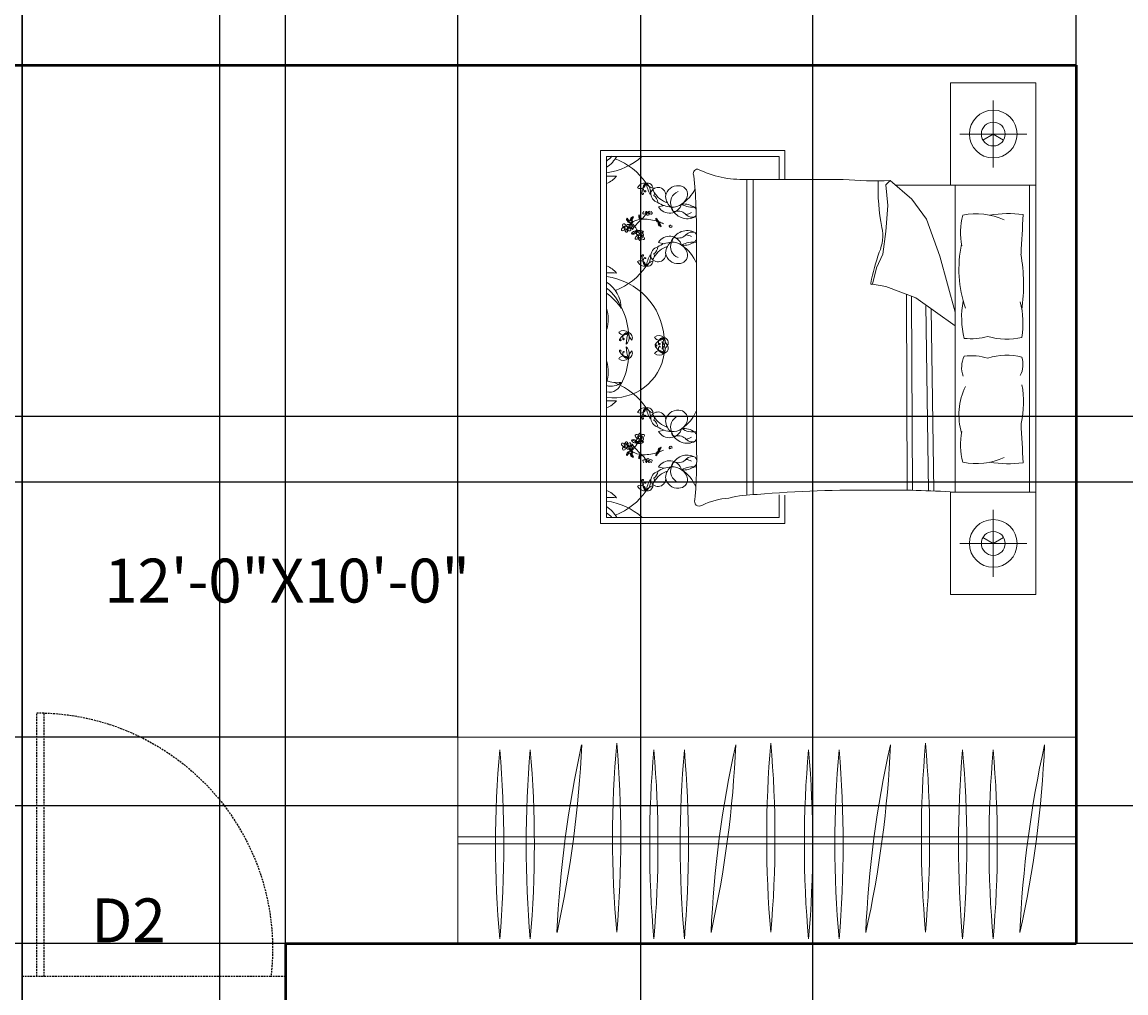
# Model space of a CAD drawing. Units: inches. Extents: x 3 to 576, y -689 to 51.
# Tile 15 of 21: x 111 to 262, y -261 to -128. Entities that reach past the tile are written whole.
import ezdxf

# ---------------------------------------------------------------- set-up
doc = ezdxf.new("R2010")
doc.units = ezdxf.units.IN
doc.header["$MEASUREMENT"] = 0
doc.linetypes.add('DASHED2', pattern=[0.375, 0.25, -0.125])
for name, color, linetype, lineweight in [('A-ANNO-DIMS', 2, 'Continuous', 18), ('A-ANNO-TEXT', 3, 'Continuous', 18), ('A-AREA-IDEN', 7, 'Continuous', 18), ('A-DOOR', 4, 'DASHED2', 25), ('A-FURN', 8, 'Continuous', 18), ('A-WALL', 7, 'Continuous', 50)]:
    doc.layers.add(name, color=color, linetype=linetype, lineweight=lineweight)
doc.styles.get("Standard").update_dxf_attribs({"font": 'arial.ttf'})
doc.dimstyles.get("Standard").update_dxf_attribs({"dimtxt": 0.18, "dimasz": 0.18, "dimexe": 0.18, "dimexo": 0.0625, "dimgap": 0.09, "dimtad": 0, "dimtih": 1, "dimtoh": 1, "dimdec": 0, "dimzin": 0, "dimdsep": 46, "dimlunit": 3, "dimtxsty": 'Standard', "dimcen": 0.09, "dimadec": 0, "dimazin": 0, "dimtfac": 1, "dimtdec": 0, "dimtofl": 0, "dimtmove": 0, "dimatfit": 3, "dimfxl": 1, "dimtolj": 1, "dimtzin": 0, "dimarcsym": 0})

# ---------------------------------------------------------------- blocks, each defined once
blk = doc.blocks.new('BED-DOUBLE')
for p, q in [((59.45, 69.91), (59.45, 0)), ((53.63, 58.35), (53.63, 67.49)), ((49.06, 62.92), (58.2, 62.92)), ((0, 60.68), (25.18, 60.68)), ((0, 9.72), (0, 60.68)), ((25.18, 60.68), (25.18, 56.73)), ((0.81, 59.87), (0.81, 10.53)), ((24.37, 59.87), (0.81, 59.87)), ((24.37, 56.73), (24.37, 59.87)), ((19.95, 13.6), (19.95, 56.73)), ((20.82, 13.66), (20.82, 56.73)), ((38.97, 55.99), (39.54, 56.55)), ((39.25, 53.16), (38.97, 55.99)), ((39.54, 56.55), (42.51, 54.01)), ((59.45, 55.93), (40.27, 55.93)), ((48.41, 55.93), (48.41, 13.98)), ((58.56, 13.98), (58.56, 55.93)), ((7.9, 52.98), (8.69, 53.14)), ((38.97, 49.62), (39.25, 53.16)), ((42.51, 54.01), (44.49, 51.31)), ((44.49, 51.31), (46.33, 46.22)), ((13.08, 20.76), (13.08, 49.15)), ((38.55, 46.5), (38.97, 49.62)), ((7.9, 48.1), (8.69, 47.94)), ((37.7, 44.66), (38.55, 46.5)), ((46.33, 46.22), (48.41, 38.59)), ((37.13, 42.39), (37.7, 44.66)), ((38.97, 42.11), (37.13, 42.39)), ((43.07, 40.55), (38.97, 42.11)), ((41.87, 14.23), (41.76, 41.05)), ((42.58, 14.23), (42.48, 40.78)), ((48.41, 36.72), (43.07, 40.55)), ((44.78, 14.2), (44.43, 39.58)), ((45.5, 14.17), (45.15, 39.06)), ((7.9, 22.3), (8.69, 22.46)), ((7.9, 17.41), (8.69, 17.26)), ((24.37, 10.53), (24.37, 13.61)), ((25.18, 13.59), (25.18, 9.72)), ((53.63, 11.56), (53.63, 2.42)), ((25.18, 9.72), (0, 9.72)), ((0.81, 10.53), (24.37, 10.53)), ((49.06, 6.99), (58.2, 6.99))]:
    blk.add_line(p, q)
for points in [[(47.8, 55.93), (47.8, 69.91), (59.45, 69.91)], [(53.63, 62.92), (52.22, 62.1)], [(53.63, 62.92), (55.04, 62.1)], [(59.45, 13.98), (47.8, 13.98), (47.8, 0), (59.45, 0)], [(53.63, 6.99), (52.22, 7.81)], [(53.63, 6.99), (55.04, 7.81)]]:
    blk.add_lwpolyline(points)
for points in [[(33.13, 56.7, 0.001242), (19.87, 56.73, -0.127202), (13.26, 58.14)], [(57.71, 51.91, 0.074897), (53.14, 51.83, -0.472817)], [(52.89, 35.28, 0.14099), (57.55, 35.14, 0.235245)], [(52.89, 32.3, -0.14099), (57.55, 32.44, -0.235245)], [(57.71, 18, -0.074897), (53.14, 18.08, 0.472817)], [(21.37, 13.68, 0.056112), (17.53, 13.18, 0.095341), (13.82, 12.19)]]:
    blk.add_lwpolyline(points, format="xyb")
for centre, radius in [((53.63, 62.92), 3.26), ((53.63, 62.92), 1.63), ((3.49, 50.11), 0.178), ((5.36, 48.94), 0.178), ((5.36, 21.45), 0.178), ((3.49, 20.29), 0.178), ((53.63, 6.99), 3.26), ((53.63, 6.99), 1.63)]:
    blk.add_circle(centre, radius)
for centre, radius, start, end in [((-2.47, 63.69), 5.54, 306.3036, 316.4814), ((-1.64, 62.09), 4.45, 303.4617, 330.1116), ((-0.42, 66.67), 9.13, 277.745, 311.8856), ((-1.32, 51.05), 9.13, 34.3865, 68.5908), ((13.3, 57.49), 0.645, 93.98, 207.3412), ((-0.61, 59.6), 3.71, 292.5547, 318.9546), ((1.38, 69.77), 12.63, 267.4081, 273.6519), ((6, 55.22), 1.01, 77.7115, 159.0387), ((5.45, 56.23), 0.762, 238.4633, 358.2869), ((7.95, 54.69), 2.31, 138.8402, 177.9352), ((6.56, 55.55), 0.747, 117.6827, 223.7762), ((6.39, 55.47), 0.757, 2.9516, 103.728), ((12.45, 57.59), 6.39, 192.5173, 207.1824), ((5.37, 55.04), 1.44, 345.4653, 54.2343), ((7.54, 57.02), 1.56, 211.3827, 255.2969), ((10.53, 54.2), 1.67, 84.9449, 172.8857), ((10.7, 54.68), 1.18, 354.4856, 91.0538), ((-59.69, 49.98), 72.78, 359.3433, 5.6887), ((37.8, 120.65), 64.12, 265.8294, 271.553), ((64.29, 55.36), 26.39, 177.4519, 191.3392), ((5.76, 54.77), 0.113, 177.9352, 11.4834), ((5.81, 54.78), 0.0551, 11.4834, 127.9409), ((6.09, 55.1), 0.0988, 223.7762, 159.7183), ((7.84, 54.58), 1.05, 350.264, 160.8688), ((8.16, 54.83), 1.31, 175.969, 254.3045), ((6.7, 54.8), 0.643, 333.9755, 53.2681), ((6.41, 53.42), 1.4, 6.1662, 51.5825), ((10.15, 56.66), 3.3, 211.2614, 251.7045), ((10.9, 54.49), 2.03, 182.3591, 234.0401), ((11.17, 53.54), 1.62, 111.5819, 201.4221), ((9.83, 55.04), 2.1, 265.2933, 346.921), ((8.16, 57.76), 5.29, 303.6671, 333.2997), ((9.88, 56.69), 3.75, 236.2883, 266.5076), ((9.4, 53.85), 1.74, 209.9085, 343.1337), ((10.13, 52.75), 0.434, 167.3041, 285.1471), ((11.31, 50.67), 2.7, 122.7011, 126.3445), ((11.81, 53.58), 2.23, 199.2822, 299.1751), ((12.57, 55.82), 2.9, 238.8218, 279.1554), ((11.31, 50.67), 2.7, 55.785, 94.7304), ((12.31, 52.24), 0.842, 30.0293, 52.325), ((3.75, 51.26), 0.199, 124.3538, 214.3923), ((4.17, 51.39), 0.538, 176.9701, 248.2913), ((8.01, 54.23), 5.2, 212.6784, 216.3746), ((4.48, 51.12), 0.464, 122.8155, 187.3992), ((4.69, 51.06), 0.538, 109.4799, 177.6828), ((4.4, 51.4), 0.199, 56.8636, 146.9021), ((4.5, 51.18), 0.206, 148.8844, 224.2646), ((8.78, 48.6), 5.2, 145.1882, 148.8844), ((5.81, 48.38), 2.9, 94.756, 119.2041), ((11.99, 44.2), 9.55, 132.2412, 142.1744), ((7.17, 51.8), 1.97, 178.3264, 187.1302), ((5.04, 51.53), 0.367, 11.3256, 64.4621), ((6.29, 52.06), 1.1, 190.2588, 210.656), ((5.55, 51.61), 0.336, 188.3432, 274.2869), ((5.84, 51.79), 0.586, 210.656, 242.6341), ((6.28, 52.3), 1.12, 218.2101, 226.3071), ((5.45, 51.35), 0.142, 325.7657, 67.4417), ((1.03, 56.11), 6.64, 313.1541, 322.0459), ((5.96, 45.49), 5.79, 73.5842, 93.8277), ((5.91, 52.13), 0.137, 142.4737, 265.053), ((6.09, 52.15), 0.294, 127.7621, 169.0403), ((5.94, 52.4), 0.414, 265.053, 338.3618), ((6.48, 51.84), 0.541, 113.4276, 137.6104), ((6.42, 52.4), 0.178, 183.2768, 356.7232), ((6.55, 52.07), 0.291, 139.7889, 227.6792), ((6.46, 51.97), 0.153, 227.6792, 350.3487), ((5.87, 52.08), 0.583, 353.0852, 15.7171), ((6.25, 52.01), 0.368, 350.3487, 43.6538), ((6.93, 52.39), 0.428, 198.7263, 262.5032), ((6.59, 52.19), 0.17, 1.1081, 91.8675), ((6.91, 52.1), 0.138, 255.2356, 54.9248), ((6.7, 52.15), 0.297, 11.5637, 52.6358), ((9.52, 51.39), 1.97, 178.3264, 187.1302), ((7.39, 51.11), 0.367, 11.3256, 64.4621), ((8.64, 51.64), 1.1, 190.2588, 210.656), ((10.62, 50.95), 1.43, 41.5653, 105.1471), ((11.41, 53.92), 2.01, 277.436, 299.9149), ((12.48, 52.59), 1.05, 221.5653, 293.8354), ((12.31, 52.24), 0.842, 314.4517, 333.558), ((58.53, 49.42), 9.37, 165.1039, 191.0369), ((51.31, 43.01), 9.01, 65.1316, 101.7583), ((723.03, 13.38), 666.43, 176.68521, 177.14978), ((2.98, 49.84), 0.137, 142.4737, 265.053), ((3.16, 49.87), 0.294, 61.2196, 169.0403), ((3, 50.12), 0.414, 265.053, 338.3618), ((3.35, 50.47), 0.351, 157.4086, 261.4386), ((3.15, 50.48), 0.176, 58.0499, 135.6268), ((3.55, 49.55), 0.541, 113.4276, 137.6104), ((3.34, 50.37), 0.118, 172.906, 277.132), ((2.95, 50.16), 0.561, 14.7558, 58.0499), ((3.62, 49.79), 0.291, 139.7889, 227.6792), ((3.74, 50.31), 0.243, 36.1046, 181.4281), ((2.93, 49.79), 0.583, 353.0852, 15.7171), ((4.04, 51.23), 0.464, 190.3057, 287.1958), ((3.31, 49.72), 0.368, 350.3487, 43.6538), ((3.59, 50.5), 0.245, 270.0645, 331.1507), ((3.8, 50.44), 0.28, 221.8413, 265.7877), ((4, 50.1), 0.428, 198.7263, 262.5032), ((3.66, 49.9), 0.17, 1.1081, 91.8675), ((3.8, 50.33), 0.174, 263.7526, 41.7054), ((3.76, 49.86), 0.297, 11.5637, 86.365), ((3.99, 51.27), 0.206, 216.3746, 291.7548), ((5.81, 48.38), 2.9, 124.0033, 132.4917), ((3.98, 49.81), 0.138, 255.2356, 54.9248), ((2.83, 48.01), 3.1, 63.7819, 68.2913), ((4.48, 50.4), 0.493, 128.3208, 208.8162), ((4.57, 50.43), 0.59, 207.7043, 254.3516), ((4.12, 50.93), 0.155, 289.3605, 111.7548), ((4.24, 50.93), 0.155, 221.8703, 44.2646), ((4.94, 50.48), 0.812, 157.2305, 229.0635), ((4.67, 50.75), 0.478, 174.4544, 220.6188), ((4.19, 50.1), 0.812, 270.278, 342.111), ((1.96, 48.08), 3.48, 30.544, 49.818), ((3.87, 50.06), 0.574, 340.0041, 40.6188), ((4.57, 50.12), 0.478, 278.7227, 324.8872), ((5.45, 49.87), 0.493, 182.8499, 266.1226), ((5.26, 50.22), 0.478, 231.7607, 277.9252), ((5.63, 50.31), 0.812, 214.5369, 286.3699), ((7.9, 51.19), 0.336, 188.3432, 274.2869), ((8.19, 51.38), 0.586, 210.656, 242.6341), ((8.64, 51.88), 1.12, 218.2101, 226.3071), ((7.81, 50.93), 0.142, 325.7657, 67.4417), ((8.21, 50.67), 0.336, 147.5332, 233.4768), ((7.94, 50.71), 0.142, 354.3784, 96.0543), ((8.51, 50.85), 0.586, 179.1859, 211.164), ((5.96, 45.49), 5.79, 63.0032, 69.8941), ((8.95, 51.12), 1.1, 211.164, 231.5612), ((9.15, 52.01), 1.97, 234.6898, 243.4936), ((9.16, 51), 1.12, 195.5129, 203.6099), ((7.9, 50.27), 0.367, 357.3579, 50.4944), ((9.48, 50.34), 0.135, 12.7051, 190.4384), ((9.56, 50.36), 0.219, 190.4384, 10.4136), ((32.84, 49.05), 5.69, 336.2616, 11.3392), ((3.53, 49.68), 0.153, 227.6792, 350.3487), ((4.73, 49.08), 0.574, 98.7227, 159.3375), ((4.44, 49.82), 0.59, 244.9899, 291.6373), ((4.49, 49.73), 0.493, 290.5253, 358.5375), ((4.85, 48.67), 0.137, 142.4737, 265.053), ((5.03, 48.7), 0.294, 61.2196, 169.0403), ((4.88, 48.95), 0.414, 265.053, 338.3618), ((5.23, 49.31), 0.351, 157.4086, 261.4386), ((5.03, 49.32), 0.176, 58.0499, 135.6268), ((5.43, 48.38), 0.541, 113.4276, 137.6104), ((5.21, 49.21), 0.118, 172.906, 277.132), ((4.83, 48.99), 0.561, 14.7558, 58.0499), ((1.96, 48.08), 3.48, 23.0501, 23.8477), ((5.5, 48.62), 0.291, 139.7889, 227.6792), ((5.4, 48.52), 0.153, 227.6792, 350.3487), ((5.4, 49.18), 0.574, 37.3105, 97.9252), ((5.61, 49.14), 0.243, 36.1046, 181.4281), ((4.81, 48.63), 0.583, 353.0852, 15.7171), ((5.47, 49.97), 0.59, 265.0106, 311.658), ((1.96, 48.08), 3.48, 357.1071, 4.7585), ((5.19, 48.56), 0.368, 350.3487, 43.6538), ((5.47, 49.33), 0.245, 270.0645, 331.1507), ((5.68, 49.27), 0.28, 221.8413, 265.7877), ((5.87, 48.94), 0.428, 198.7263, 262.5032), ((5.53, 48.74), 0.17, 1.1081, 91.8675), ((5.68, 49.17), 0.174, 263.7526, 41.7054), ((5.64, 48.7), 0.297, 11.5637, 86.365), ((5.85, 48.65), 0.138, 255.2356, 54.9248), ((9.4, 47.23), 1.74, 16.8663, 150.0915), ((10.13, 48.33), 0.434, 74.8529, 192.6959), ((11.81, 47.5), 2.23, 60.8249, 160.7178), ((10.62, 50.13), 1.43, 254.8529, 318.4347), ((11.41, 47.16), 2.01, 60.0851, 82.564), ((12.48, 48.49), 1.05, 66.1646, 138.4347), ((12.31, 48.84), 0.842, 307.675, 336.7144), ((12.31, 48.84), 0.842, 23.229, 45.5483), ((8.16, 46.25), 1.31, 105.6955, 184.031), ((6.41, 47.66), 1.4, 308.4175, 353.8338), ((10.15, 44.42), 3.3, 108.2955, 148.7386), ((9.88, 44.39), 3.75, 93.4924, 123.7117), ((10.9, 46.59), 2.03, 125.9599, 177.6409), ((11.17, 47.54), 1.62, 158.5779, 248.4181), ((9.83, 46.04), 2.1, 13.079, 94.7067), ((11.31, 50.41), 2.7, 233.6555, 237.2989), ((12.57, 45.26), 2.9, 79.7133, 121.1782), ((11.31, 50.41), 2.7, 265.2696, 304.215), ((8.16, 43.32), 5.29, 21.4941, 56.3329), ((63.55, 37.54), 27.11, 160.1194, 169.3383), ((65.19, 44.49), 16.25, 168.0397, 199.2615), ((5.45, 44.85), 0.762, 1.7131, 121.5367), ((6, 45.86), 1.01, 200.9613, 282.2885), ((5.76, 46.31), 0.113, 348.5166, 182.0648), ((7.95, 46.39), 2.31, 182.0648, 221.1598), ((5.81, 46.3), 0.0551, 232.0591, 348.5166), ((6.56, 45.54), 0.747, 136.2238, 242.3173), ((6.13, 45.97), 0.0595, 200.2667, 136.2271), ((5.37, 46.05), 1.44, 305.7657, 14.5347), ((12.45, 43.49), 6.39, 152.8176, 167.4827), ((6.39, 45.61), 0.757, 256.272, 357.0484), ((7.54, 44.06), 1.56, 104.7031, 148.6173), ((7.84, 46.5), 1.05, 199.1312, 9.736), ((6.7, 46.28), 0.643, 306.7319, 26.0245), ((10.53, 46.88), 1.67, 187.1143, 275.0551), ((10.7, 46.4), 1.18, 268.9462, 5.5144), ((32.41, 42.33), 25.35, 352.2196, 9.497), ((-0.61, 41.48), 3.71, 41.0454, 67.4453), ((1.38, 31.32), 12.63, 86.3481, 92.5919), ((-1.32, 50.03), 9.13, 291.4092, 325.6135), ((-0.42, 34.41), 9.13, 4.4623, 82.255), ((-1.64, 38.99), 4.45, 1.272, 56.5383), ((37.07, 42.55), 0.169, 178.8623, 289.7536), ((-2.47, 37.39), 5.54, 17.8504, 53.6964), ((-4.03, 34.48), 8.25, 34.0123, 54.053), ((-5.31, 35.11), 9.13, 4.4623, 27.4146), ((61.64, 37.91), 12.33, 169.8617, 193.6238), ((45.23, 36.98), 12.46, 351.5249, 13.96), ((-3.99, 37.66), 5.02, 343.5431, 17.0202), ((-6.58, 35.67), 7.42, 4.3787, 5.6357), ((-11.66, 31.77), 13.27, 19.7217, 19.9028), ((3.11, 35.07), 1.01, 47.7873, 129.1145), ((3.14, 36.22), 0.762, 208.5391, 328.3627), ((2.68, 34.8), 0.113, 148.011, 341.5592), ((4.54, 33.64), 2.31, 108.9159, 148.011), ((2.73, 34.78), 0.0551, 341.5592, 98.0167), ((3.76, 35.07), 0.747, 87.7585, 193.852), ((3.13, 34.92), 0.0988, 193.852, 129.9245), ((9.89, 33.91), 6.39, 162.593, 177.2582), ((2.48, 35.23), 1.44, 315.5411, 24.3101), ((5.35, 35.86), 1.56, 181.4585, 225.3727), ((3.58, 35.09), 0.757, 333.0274, 73.8037), ((8, 34.37), 1.01, 47.7873, 129.1145), ((8.03, 35.52), 0.762, 208.5391, 328.3627), ((9.43, 32.94), 2.31, 108.9159, 148.011), ((8.65, 34.38), 0.747, 87.7585, 193.852), ((7.37, 34.53), 1.44, 315.5411, 24.3101), ((14.78, 33.21), 6.39, 162.593, 177.2582), ((8.47, 34.4), 0.757, 333.0274, 73.8037), ((10.24, 35.16), 1.56, 181.4585, 225.3727), ((50.55, 43.52), 8.57, 264.0129, 285.8293), ((2.68, 33.27), 0.113, 18.4408, 211.989), ((4.54, 34.43), 2.31, 211.989, 251.0841), ((2.73, 33.29), 0.0551, 261.9833, 18.4408), ((3.76, 32.99), 0.747, 166.148, 272.2415), ((3.17, 33.16), 0.0595, 230.1909, 166.0209), ((9.89, 34.16), 6.39, 182.7418, 197.407), ((2.48, 32.84), 1.44, 335.6899, 44.4589), ((5.35, 32.21), 1.56, 134.6273, 178.5415), ((3.58, 32.97), 0.757, 286.1963, 26.9726), ((8.03, 32.55), 0.762, 31.6373, 151.4609), ((7.57, 34.1), 0.113, 148.011, 341.5592), ((7.57, 33.97), 0.113, 18.4408, 211.989), ((9.43, 35.13), 2.31, 211.989, 251.0841), ((7.62, 34.08), 0.0551, 341.5592, 98.0167), ((7.62, 33.99), 0.0551, 261.9833, 18.4408), ((8.65, 33.69), 0.747, 166.148, 272.2415), ((8.02, 34.22), 0.0988, 193.852, 129.9245), ((8.06, 33.86), 0.0595, 230.1909, 166.0209), ((7.37, 33.54), 1.44, 335.6899, 44.4589), ((14.78, 34.86), 6.39, 182.7418, 197.407), ((8.47, 33.67), 0.757, 286.1963, 26.9726), ((10.24, 32.91), 1.56, 134.6273, 178.5415), ((1.69, 33.95), 7.07, 262.8636, 351.8197), ((-3.99, 30.4), 5.02, 342.9798, 16.4569), ((-6.58, 32.39), 7.42, 354.3643, 355.6213), ((-11.66, 36.3), 13.27, 340.0972, 340.2783), ((3.14, 31.85), 0.762, 31.6373, 151.4609), ((3.11, 33), 1.01, 230.8855, 312.2127), ((-5.31, 32.96), 9.13, 332.5854, 355.5377), ((8, 33.7), 1.01, 230.8855, 312.2127), ((53.02, 31.01), 3.71, 155.0183, 198.5407), ((50.55, 24.06), 8.57, 74.1707, 95.9871), ((54.23, 31.48), 3.46, 333.3437, 16.1026), ((2.33, 33.04), 4.09, 248.117, 276.6195), ((1.2, 29.29), 1.64, 256.3898, 349.0739), ((1.42, 30.52), 2.07, 252.8609, 311.9049), ((-1.32, 20.37), 9.13, 34.3865, 68.5908), ((45.48, 26.29), 12.29, 346.3427, 11.1841), ((57.84, 24.53), 8.9, 153.8761, 196.1746), ((1.38, 39.08), 12.63, 267.4081, 273.6519), ((-0.61, 28.92), 3.71, 292.5547, 318.9546), ((6, 24.53), 1.01, 77.7115, 159.0387), ((5.45, 25.55), 0.762, 238.4633, 358.2869), ((7.95, 24), 2.31, 138.8402, 177.9352), ((5.81, 24.09), 0.0551, 11.4834, 127.9409), ((6.56, 24.86), 0.747, 117.6827, 223.7762), ((6.09, 24.41), 0.0988, 223.7762, 159.7183), ((6.39, 24.79), 0.757, 2.9516, 103.728), ((7.54, 26.34), 1.56, 211.3827, 255.2969), ((5.37, 24.35), 1.44, 345.4653, 54.2343), ((12.45, 26.91), 6.39, 192.5173, 207.1824), ((7.84, 23.9), 1.05, 350.264, 160.8688), ((8.16, 24.15), 1.31, 175.969, 254.3045), ((6.7, 24.12), 0.643, 333.9755, 53.2681), ((10.15, 25.98), 3.3, 211.2614, 251.7045), ((10.53, 23.52), 1.67, 84.9449, 172.8857), ((11.17, 22.86), 1.62, 111.5819, 201.4221), ((10.7, 24), 1.18, 354.4856, 91.0538), ((8.16, 27.08), 5.29, 303.6671, 338.5059), ((5.76, 24.08), 0.113, 177.9352, 11.4834), ((6.41, 22.74), 1.4, 6.1662, 51.5825), ((9.88, 26.01), 3.75, 236.2883, 266.5076), ((9.4, 23.17), 1.74, 209.9085, 343.1337), ((10.9, 23.81), 2.03, 182.3591, 234.0401), ((9.83, 24.36), 2.1, 265.2933, 346.921), ((12.57, 25.14), 2.9, 238.8218, 280.2867), ((11.31, 19.99), 2.7, 55.785, 94.7304), ((723.03, 56.53), 666.43, 182.85022, 183.31479), ((4.44, 20.58), 0.59, 68.3627, 115.0101), ((4.19, 20.3), 0.812, 17.889, 89.722), ((4.73, 21.32), 0.574, 200.6625, 261.2773), ((4.49, 20.66), 0.493, 1.4625, 69.4747), ((4.85, 21.72), 0.137, 94.947, 217.5263), ((5.03, 21.7), 0.294, 190.9597, 298.7804), ((4.88, 21.45), 0.414, 21.6382, 94.947), ((5.23, 21.09), 0.351, 98.5614, 202.5914), ((5.43, 22.01), 0.541, 222.3896, 246.5724), ((5.21, 21.19), 0.118, 82.868, 187.094), ((4.83, 21.41), 0.561, 301.9501, 345.2442), ((5.5, 21.78), 0.291, 132.3208, 220.2111), ((5.4, 21.88), 0.153, 9.6513, 132.3208), ((4.81, 21.77), 0.583, 344.2829, 6.9148), ((5.61, 21.26), 0.243, 178.5719, 323.8954), ((1.96, 22.32), 3.48, 355.2415, 2.8929), ((5.19, 21.84), 0.368, 316.3462, 9.6513), ((5.87, 21.46), 0.428, 97.4968, 161.2737), ((5.68, 21.12), 0.28, 94.2123, 138.1587), ((5.47, 21.07), 0.245, 28.8493, 89.9355), ((5.53, 21.66), 0.17, 268.1325, 358.8919), ((5.64, 21.7), 0.297, 273.635, 348.4363), ((5.68, 21.23), 0.174, 318.2946, 96.2474), ((5.85, 21.75), 0.138, 305.0752, 104.7644), ((10.13, 22.07), 0.434, 167.3041, 285.1471), ((11.31, 19.99), 2.7, 122.7011, 126.3445), ((11.81, 22.9), 2.23, 199.2822, 299.1751), ((10.62, 20.26), 1.43, 41.5653, 105.1471), ((11.41, 23.23), 2.01, 277.436, 299.9149), ((12.48, 21.91), 1.05, 221.5653, 293.8354), ((12.31, 21.55), 0.842, 23.2856, 52.325), ((12.31, 21.55), 0.842, 314.4517, 336.7144), ((58.53, 20.49), 9.37, 168.9631, 194.8961), ((2.98, 20.56), 0.137, 94.947, 217.5263), ((3.16, 20.53), 0.294, 190.9597, 298.7804), ((3, 20.28), 0.414, 21.6382, 94.947), ((3.35, 19.93), 0.351, 98.5614, 202.5914), ((3.15, 19.91), 0.176, 224.3732, 301.9501), ((3.55, 20.85), 0.541, 222.3896, 246.5724), ((3.34, 20.03), 0.118, 82.868, 187.094), ((2.95, 20.24), 0.561, 301.9501, 345.2442), ((3.62, 20.61), 0.291, 132.3208, 220.2111), ((3.53, 20.71), 0.153, 9.6513, 132.3208), ((2.93, 20.61), 0.583, 344.2829, 6.9148), ((3.74, 20.09), 0.243, 178.5719, 323.8954), ((3.31, 20.68), 0.368, 316.3462, 9.6513), ((4.04, 19.17), 0.464, 72.8042, 169.6943), ((4, 20.3), 0.428, 97.4968, 161.2737), ((3.8, 19.96), 0.28, 94.2123, 138.1587), ((3.59, 19.9), 0.245, 28.8493, 89.9355), ((3.66, 20.5), 0.17, 268.1325, 358.8919), ((3.76, 20.54), 0.297, 273.635, 348.4363), ((3.8, 20.07), 0.174, 318.2946, 96.2474), ((5.81, 22.02), 2.9, 227.5083, 235.9967), ((3.98, 20.59), 0.138, 305.0752, 104.7644), ((2.83, 22.39), 3.1, 291.7087, 296.2181), ((4.48, 20), 0.493, 151.1838, 231.6792), ((4.57, 19.96), 0.59, 105.6484, 152.2957), ((4.12, 19.47), 0.155, 248.2452, 70.6395), ((4.94, 19.92), 0.812, 130.9365, 202.7695), ((4.24, 19.47), 0.155, 315.7354, 138.1297), ((4.67, 19.65), 0.478, 139.3812, 185.5456), ((1.96, 22.32), 3.48, 310.182, 329.456), ((3.87, 20.33), 0.574, 319.3812, 19.9959), ((11.99, 26.2), 9.55, 217.8256, 227.7588), ((4.57, 20.28), 0.478, 35.1128, 81.2773), ((5.03, 21.08), 0.176, 224.3732, 301.9501), ((5.45, 20.52), 0.493, 93.8774, 177.1501), ((5.63, 20.09), 0.812, 73.6301, 145.4631), ((5.26, 20.18), 0.478, 82.0748, 128.2393), ((1.96, 22.32), 3.48, 336.1523, 336.9499), ((5.4, 21.22), 0.574, 262.0748, 322.6895), ((5.47, 20.43), 0.59, 48.342, 94.9894), ((8.21, 19.72), 0.336, 126.5232, 212.4668), ((8.51, 19.55), 0.586, 148.836, 180.8141), ((7.94, 19.68), 0.142, 263.9457, 5.6216), ((5.96, 24.9), 5.79, 290.1059, 296.9968), ((8.95, 19.28), 1.1, 128.4388, 148.836), ((9.15, 18.38), 1.97, 116.5064, 125.3102), ((9.16, 19.4), 1.12, 156.3901, 164.4871), ((7.9, 20.13), 0.367, 309.5056, 2.6421), ((9.56, 20.04), 0.219, 349.5864, 169.5616), ((9.48, 20.06), 0.135, 169.5616, 347.2949), ((-54.91, 18.62), 68.03, 355.2402, 1.8035), ((3.75, 19.14), 0.199, 145.6077, 235.6462), ((4.17, 19.01), 0.538, 111.7087, 183.0299), ((8.01, 16.17), 5.2, 143.6254, 147.3216), ((3.99, 19.13), 0.206, 68.2452, 143.6254), ((4.48, 19.27), 0.464, 172.6008, 237.1845), ((4.69, 19.33), 0.538, 182.3172, 250.5201), ((4.4, 18.99), 0.199, 213.0979, 303.1364), ((4.5, 19.21), 0.206, 135.7354, 211.1156), ((8.78, 21.8), 5.2, 211.1156, 214.8118), ((5.81, 22.02), 2.9, 240.7959, 265.244), ((6.29, 18.34), 1.1, 149.344, 169.7412), ((7.17, 18.6), 1.97, 172.8698, 181.6736), ((5.04, 18.87), 0.367, 295.5379, 348.6744), ((5.55, 18.79), 0.336, 85.7131, 171.6568), ((5.84, 18.61), 0.586, 117.3659, 149.344), ((6.28, 18.1), 1.12, 133.6929, 141.7899), ((5.45, 19.05), 0.142, 292.5583, 34.2343), ((5.96, 24.9), 5.79, 266.1723, 286.4158), ((1.03, 14.28), 6.64, 37.9541, 46.8459), ((5.91, 18.27), 0.137, 94.947, 217.5263), ((6.09, 18.24), 0.294, 190.9597, 232.2379), ((5.94, 18), 0.414, 21.6382, 94.947), ((6.48, 18.56), 0.541, 222.3896, 246.5724), ((6.42, 18), 0.178, 3.2768, 176.7232), ((6.55, 18.32), 0.291, 132.3208, 220.2111), ((6.46, 18.43), 0.153, 9.6513, 132.3208), ((5.87, 18.32), 0.583, 344.2829, 6.9148), ((6.25, 18.39), 0.368, 316.3462, 9.6513), ((6.93, 18.01), 0.428, 97.4968, 161.2737), ((6.59, 18.21), 0.17, 268.1325, 358.8919), ((6.91, 18.3), 0.138, 305.0752, 104.7644), ((6.7, 18.25), 0.297, 307.3642, 348.4363), ((8.64, 18.76), 1.1, 149.344, 169.7412), ((9.52, 19.01), 1.97, 172.8698, 181.6736), ((7.39, 19.29), 0.367, 295.5379, 348.6744), ((7.9, 19.21), 0.336, 85.7131, 171.6568), ((8.19, 19.02), 0.586, 117.3659, 149.344), ((8.64, 18.52), 1.12, 133.6929, 141.7899), ((7.81, 19.46), 0.142, 292.5583, 34.2343), ((9.4, 16.55), 1.74, 16.8663, 150.0915), ((11.81, 16.82), 2.23, 60.8249, 160.7178), ((10.62, 19.45), 1.43, 254.8529, 318.4347), ((11.41, 16.48), 2.01, 60.0851, 82.564), ((12.48, 17.81), 1.05, 66.1646, 138.4347), ((12.31, 18.16), 0.842, 16.6343, 45.5483), ((51.31, 26.9), 9.01, 258.2417, 294.8684), ((8.16, 15.56), 1.31, 105.6955, 184.031), ((6.41, 16.98), 1.4, 308.4175, 353.8338), ((10.15, 13.74), 3.3, 108.2955, 148.7386), ((9.88, 13.7), 3.75, 93.4924, 123.7117), ((10.9, 15.91), 2.03, 125.9599, 177.6409), ((11.17, 16.86), 1.62, 158.5779, 248.4181), ((9.83, 15.35), 2.1, 13.079, 94.7067), ((10.13, 17.65), 0.434, 74.8529, 192.6959), ((11.31, 19.72), 2.7, 233.6555, 237.2989), ((12.57, 14.57), 2.9, 79.249, 121.1782), ((11.31, 19.72), 2.7, 265.2696, 304.215), ((8.16, 12.63), 5.29, 23.6453, 56.3329), ((12.31, 18.16), 0.842, 307.675, 342.5814), ((5.76, 15.63), 0.113, 348.5166, 182.0648), ((7.95, 15.71), 2.31, 182.0648, 221.1598), ((5.81, 15.62), 0.0551, 232.0591, 348.5166), ((6.56, 14.85), 0.747, 136.2238, 242.3173), ((6.13, 15.29), 0.0595, 200.2667, 136.2271), ((12.45, 12.81), 6.39, 152.8176, 167.4827), ((5.37, 15.36), 1.44, 305.7657, 14.5347), ((7.84, 15.82), 1.05, 199.1312, 9.736), ((6.7, 15.6), 0.643, 306.7319, 26.0245), ((10.53, 16.2), 1.67, 187.1143, 275.0551), ((10.7, 15.72), 1.18, 268.9462, 5.5144), ((-0.61, 10.8), 3.71, 41.0454, 67.4453), ((-1.32, 19.35), 9.13, 291.4092, 325.6135), ((5.45, 14.17), 0.762, 1.7131, 121.5367), ((6, 15.18), 1.01, 200.9613, 282.2885), ((7.54, 13.38), 1.56, 104.7031, 148.6173), ((6.39, 14.93), 0.757, 256.272, 357.0484), ((35.29, -149.59), 163.86, 89.1145, 94.8735), ((39.86, -111.34), 125.62, 86.1, 90.9282), ((1.38, 0.63), 12.63, 86.3481, 92.5919), ((-0.42, 3.73), 9.13, 48.1144, 82.255), ((13.47, 12.72), 0.637, 156.5219, 303.8264), ((-1.64, 8.31), 4.45, 29.8884, 56.5383), ((-2.47, 6.71), 5.54, 43.5186, 53.6964)]:
    blk.add_arc(centre, radius, start, end)
blk = doc.blocks.new('DOOR-900')
for p, q in [((34, 36), (0, 36)), ((2, 36), (2, 0)), ((36, 36), (34, 36))]:
    blk.add_line(p, q)
blk.add_arc((2, 32.22), 32.22, 270, 6.7329)
blk = doc.blocks.new('*D65')
at = {"layer": 'A-ANNO-DIMS', "color": 0, "lineweight": -2, "transparency": 16777216}
for p, q in [((531.23, -50.31), (2.66, -50.31)), ((2.84, -50.49), (2.84, -116.13)), ((2.84, -182.13), (2.84, -116.49)), ((531.23, -182.31), (2.66, -182.31))]:
    blk.add_line(p, q, dxfattribs=at)
at = {"layer": 'A-ANNO-DIMS', "color": 0, "transparency": 16777216}
for points in [[(2.81, -50.49), (2.87, -50.49), (2.84, -50.31)], [(2.81, -182.13), (2.87, -182.13), (2.84, -182.31)]]:
    blk.add_solid(points, dxfattribs=at)
at = {"layer": 'Defpoints', "color": 0, "transparency": 16777216}
for p in [(531.29, -50.31), (2.84, -182.31), (531.29, -182.31)]:
    blk.add_point(p, dxfattribs=at)
at = {"layer": 'A-ANNO-DIMS', "color": 0, "transparency": 16777216, "insert": (2.84, -116.31), "char_height": 0.18, "attachment_point": 5}
blk.add_mtext('\\A1;11\'-0"', dxfattribs=at)
blk = doc.blocks.new('*D66')
at = {"layer": 'A-ANNO-DIMS', "color": 0, "lineweight": -2, "transparency": 16777216}
for p, q in [((531.23, -182.31), (2.66, -182.31)), ((2.84, -182.49), (2.84, -186.63)), ((2.84, -191.13), (2.84, -186.99)), ((531.23, -191.31), (2.66, -191.31))]:
    blk.add_line(p, q, dxfattribs=at)
at = {"layer": 'A-ANNO-DIMS', "color": 0, "transparency": 16777216}
for points in [[(2.81, -182.49), (2.87, -182.49), (2.84, -182.31)], [(2.81, -191.13), (2.87, -191.13), (2.84, -191.31)]]:
    blk.add_solid(points, dxfattribs=at)
at = {"layer": 'Defpoints', "color": 0, "transparency": 16777216}
for p in [(531.29, -182.31), (2.84, -191.31), (531.29, -191.31)]:
    blk.add_point(p, dxfattribs=at)
at = {"layer": 'A-ANNO-DIMS', "color": 0, "transparency": 16777216, "insert": (2.84, -186.81), "char_height": 0.18, "attachment_point": 5}
blk.add_mtext('\\A1;0\'-9"', dxfattribs=at)
blk = doc.blocks.new('*D67')
at = {"layer": 'A-ANNO-DIMS', "color": 0, "lineweight": -2, "transparency": 16777216}
for p, q in [((531.23, -191.31), (2.66, -191.31)), ((2.84, -191.49), (2.84, -222.63)), ((2.84, -254.13), (2.84, -222.99)), ((531.23, -254.31), (2.66, -254.31))]:
    blk.add_line(p, q, dxfattribs=at)
at = {"layer": 'A-ANNO-DIMS', "color": 0, "transparency": 16777216}
for points in [[(2.81, -191.49), (2.87, -191.49), (2.84, -191.31)], [(2.81, -254.13), (2.87, -254.13), (2.84, -254.31)]]:
    blk.add_solid(points, dxfattribs=at)
at = {"layer": 'Defpoints', "color": 0, "transparency": 16777216}
for p in [(531.29, -191.31), (2.84, -254.31), (531.29, -254.31)]:
    blk.add_point(p, dxfattribs=at)
at = {"layer": 'A-ANNO-DIMS', "color": 0, "transparency": 16777216, "insert": (2.84, -222.81), "char_height": 0.18, "attachment_point": 5}
blk.add_mtext('\\A1;5\'-3"', dxfattribs=at)
blk = doc.blocks.new('*D68')
at = {"layer": 'A-ANNO-DIMS', "color": 0, "lineweight": -2, "transparency": 16777216}
for p, q in [((531.23, -254.31), (2.66, -254.31)), ((2.84, -254.49), (2.84, -258.63)), ((2.84, -263.13), (2.84, -258.99)), ((531.23, -263.31), (2.66, -263.31))]:
    blk.add_line(p, q, dxfattribs=at)
at = {"layer": 'A-ANNO-DIMS', "color": 0, "transparency": 16777216}
for points in [[(2.81, -254.49), (2.87, -254.49), (2.84, -254.31)], [(2.81, -263.13), (2.87, -263.13), (2.84, -263.31)]]:
    blk.add_solid(points, dxfattribs=at)
at = {"layer": 'Defpoints', "color": 0, "transparency": 16777216}
for p in [(531.29, -254.31), (2.84, -263.31), (531.29, -263.31)]:
    blk.add_point(p, dxfattribs=at)
at = {"layer": 'A-ANNO-DIMS', "color": 0, "transparency": 16777216, "insert": (2.84, -258.81), "char_height": 0.18, "attachment_point": 5}
blk.add_mtext('\\A1;0\'-9"', dxfattribs=at)
blk = doc.blocks.new('*D86')
at = {"layer": 'A-ANNO-DIMS', "color": 0, "lineweight": -2, "transparency": 16777216}
for p, q in [((111.29, -97.21), (111.29, -688.94)), ((195.78, -97.21), (195.78, -688.94)), ((111.47, -688.76), (153, -688.76)), ((195.6, -688.76), (154.08, -688.76))]:
    blk.add_line(p, q, dxfattribs=at)
at = {"layer": 'A-ANNO-DIMS', "color": 0, "transparency": 16777216}
for points in [[(111.47, -688.73), (111.47, -688.79), (111.29, -688.76)], [(195.6, -688.73), (195.6, -688.79), (195.78, -688.76)]]:
    blk.add_solid(points, dxfattribs=at)
at = {"layer": 'Defpoints', "color": 0, "transparency": 16777216}
for p in [(111.29, -97.15), (195.78, -97.15), (195.78, -688.76)]:
    blk.add_point(p, dxfattribs=at)
at = {"layer": 'A-ANNO-DIMS', "color": 0, "transparency": 16777216, "insert": (153.54, -688.76), "char_height": 0.18, "attachment_point": 5}
blk.add_mtext('\\A1;7\'-0 1/2"', dxfattribs=at)
blk = doc.blocks.new('*D88')
at = {"layer": 'A-ANNO-DIMS', "color": 0, "lineweight": -2, "transparency": 16777216}
for p, q in [((170.8, -226.08), (170.8, 51.32)), ((255.29, -226.08), (255.29, 51.32)), ((170.98, 51.14), (212.51, 51.14)), ((255.11, 51.14), (213.59, 51.14))]:
    blk.add_line(p, q, dxfattribs=at)
at = {"layer": 'A-ANNO-DIMS', "color": 0, "transparency": 16777216}
for points in [[(170.98, 51.17), (170.98, 51.11), (170.8, 51.14)], [(255.11, 51.17), (255.11, 51.11), (255.29, 51.14)]]:
    blk.add_solid(points, dxfattribs=at)
at = {"layer": 'Defpoints', "color": 0, "transparency": 16777216}
for p in [(255.29, 51.14), (170.8, -226.15), (255.29, -226.15)]:
    blk.add_point(p, dxfattribs=at)
at = {"layer": 'A-ANNO-DIMS', "color": 0, "transparency": 16777216, "insert": (213.05, 51.14), "char_height": 0.18, "attachment_point": 5}
blk.add_mtext('\\A1;7\'-0 1/2"', dxfattribs=at)
blk = doc.blocks.new('*D89')
at = {"layer": 'A-ANNO-DIMS', "color": 0, "lineweight": -2, "transparency": 16777216}
for p, q in [((170.74, -226.15), (2.66, -226.15)), ((2.84, -226.33), (2.84, -240.05)), ((2.84, -254.13), (2.84, -240.41)), ((170.74, -254.31), (2.66, -254.31))]:
    blk.add_line(p, q, dxfattribs=at)
at = {"layer": 'A-ANNO-DIMS', "color": 0, "transparency": 16777216}
for points in [[(2.81, -226.33), (2.87, -226.33), (2.84, -226.15)], [(2.81, -254.13), (2.87, -254.13), (2.84, -254.31)]]:
    blk.add_solid(points, dxfattribs=at)
at = {"layer": 'Defpoints', "color": 0, "transparency": 16777216}
for p in [(2.84, -226.15), (170.8, -226.15), (170.8, -254.31)]:
    blk.add_point(p, dxfattribs=at)
at = {"layer": 'A-ANNO-DIMS', "color": 0, "transparency": 16777216, "insert": (2.84, -240.23), "char_height": 0.18, "attachment_point": 5}
blk.add_mtext('\\A1;2\'-4"', dxfattribs=at)
blk = doc.blocks.new('*D114')
at = {"layer": 'A-ANNO-DIMS', "color": 0, "lineweight": -2, "transparency": 16777216}
for p, q in [((147.29, -377.25), (147.29, 51.32)), ((219.29, -377.25), (219.29, 51.32)), ((147.47, 51.14), (182.96, 51.14)), ((219.11, 51.14), (183.62, 51.14))]:
    blk.add_line(p, q, dxfattribs=at)
at = {"layer": 'A-ANNO-DIMS', "color": 0, "transparency": 16777216}
for points in [[(147.47, 51.17), (147.47, 51.11), (147.29, 51.14)], [(219.11, 51.17), (219.11, 51.11), (219.29, 51.14)]]:
    blk.add_solid(points, dxfattribs=at)
at = {"layer": 'Defpoints', "color": 0, "transparency": 16777216}
for p in [(219.29, 51.14), (147.29, -377.31), (219.29, -377.31)]:
    blk.add_point(p, dxfattribs=at)
at = {"layer": 'A-ANNO-DIMS', "color": 0, "transparency": 16777216, "insert": (183.29, 51.14), "char_height": 0.18, "attachment_point": 5}
blk.add_mtext('\\A1;6\'-0"', dxfattribs=at)
blk = doc.blocks.new('*D119')
at = {"layer": 'A-ANNO-DIMS', "color": 0, "lineweight": -2, "transparency": 16777216}
for p, q in [((47.29, -311.25), (47.29, 51.32)), ((111.29, -311.25), (111.29, 51.32)), ((47.47, 51.14), (78.96, 51.14)), ((111.11, 51.14), (79.62, 51.14))]:
    blk.add_line(p, q, dxfattribs=at)
at = {"layer": 'A-ANNO-DIMS', "color": 0, "transparency": 16777216}
for points in [[(47.47, 51.17), (47.47, 51.11), (47.29, 51.14)], [(111.11, 51.17), (111.11, 51.11), (111.29, 51.14)]]:
    blk.add_solid(points, dxfattribs=at)
at = {"layer": 'Defpoints', "color": 0, "transparency": 16777216}
for p in [(111.29, 51.14), (47.29, -311.31), (111.29, -311.31)]:
    blk.add_point(p, dxfattribs=at)
at = {"layer": 'A-ANNO-DIMS', "color": 0, "transparency": 16777216, "insert": (79.29, 51.14), "char_height": 0.18, "attachment_point": 5}
blk.add_mtext('\\A1;5\'-4"', dxfattribs=at)
blk = doc.blocks.new('*D120')
at = {"layer": 'A-ANNO-DIMS', "color": 0, "lineweight": -2, "transparency": 16777216}
for p, q in [((111.29, -302.25), (111.29, 51.32)), ((138.29, -302.25), (138.29, 51.32)), ((111.47, 51.14), (124.46, 51.14)), ((138.11, 51.14), (125.12, 51.14))]:
    blk.add_line(p, q, dxfattribs=at)
at = {"layer": 'A-ANNO-DIMS', "color": 0, "transparency": 16777216}
for points in [[(111.47, 51.17), (111.47, 51.11), (111.29, 51.14)], [(138.11, 51.17), (138.11, 51.11), (138.29, 51.14)]]:
    blk.add_solid(points, dxfattribs=at)
at = {"layer": 'Defpoints', "color": 0, "transparency": 16777216}
for p in [(138.29, 51.14), (111.29, -302.31), (138.29, -302.31)]:
    blk.add_point(p, dxfattribs=at)
at = {"layer": 'A-ANNO-DIMS', "color": 0, "transparency": 16777216, "insert": (124.79, 51.14), "char_height": 0.18, "attachment_point": 5}
blk.add_mtext('\\A1;2\'-3"', dxfattribs=at)
blk = doc.blocks.new('*D123')
at = {"layer": 'A-ANNO-DIMS', "color": 0, "lineweight": -2, "transparency": 16777216}
for p, q in [((513.55, -235.5), (2.66, -235.5)), ((2.84, -235.68), (2.84, -244.72)), ((2.84, -254.13), (2.84, -245.08)), ((531.23, -254.31), (2.66, -254.31))]:
    blk.add_line(p, q, dxfattribs=at)
at = {"layer": 'A-ANNO-DIMS', "color": 0, "transparency": 16777216}
for points in [[(2.81, -235.68), (2.87, -235.68), (2.84, -235.5)], [(2.81, -254.13), (2.87, -254.13), (2.84, -254.31)]]:
    blk.add_solid(points, dxfattribs=at)
at = {"layer": 'Defpoints', "color": 0, "transparency": 16777216}
for p in [(513.61, -235.5), (2.84, -254.31), (531.29, -254.31)]:
    blk.add_point(p, dxfattribs=at)
at = {"layer": 'A-ANNO-DIMS', "color": 0, "transparency": 16777216, "insert": (2.84, -244.9), "char_height": 0.18, "attachment_point": 5}
blk.add_mtext('\\A1;1\'-7"', dxfattribs=at)

msp = doc.modelspace()

# ---------------------------------------------------------------- linework, layer by layer
at = {"layer": 'A-DOOR'}
msp.add_line((114.29, -258.81), (114.29, -222.81), dxfattribs=at)
at = {"layer": 'A-FURN'}
for p, q in [((255.29, -226.15), (170.8, -226.15)), ((170.8, -226.15), (170.8, -254.31)), ((255.29, -226.15), (255.29, -254.31)), ((255.29, -239.76), (170.8, -239.76)), ((255.29, -240.7), (170.8, -240.7)), ((255.29, -254.31), (170.8, -254.31))]:
    msp.add_line(p, q, dxfattribs=at)
for centre, start, end in [((39.68, -220.74), 347.508, 357.5023), ((332.4, -259.25), 167.508, 177.5023), ((340.14, -239.88), 175.0028, 184.9972), ((44.89, -239.88), 355.0028, 4.9972), ((60.73, -220.74), 347.508, 357.5023), ((353.45, -259.25), 167.508, 177.5023), ((361.19, -239.88), 175.0028, 184.9972), ((65.94, -239.88), 355.0028, 4.9972), ((374.58, -259.25), 167.508, 177.5023), ((81.86, -220.74), 347.508, 357.5023), ((382.32, -239.88), 175.0028, 184.9972), ((87.07, -239.88), 355.0028, 4.9972), ((395.63, -259.25), 167.508, 177.5023), ((102.91, -220.74), 347.508, 357.5023), ((324.16, -240.79), 175.0028, 184.9972), ((28.91, -240.79), 355.0028, 4.9972), ((328.33, -240.79), 175.0028, 184.9972), ((33.08, -240.79), 355.0028, 4.9972), ((345.21, -240.79), 175.0028, 184.9972), ((49.96, -240.79), 355.0028, 4.9972), ((349.38, -240.79), 175.0028, 184.9972), ((54.13, -240.79), 355.0028, 4.9972), ((366.34, -240.79), 175.0028, 184.9972), ((71.09, -240.79), 355.0028, 4.9972), ((370.51, -240.79), 175.0028, 184.9972), ((75.26, -240.79), 355.0028, 4.9972), ((387.39, -240.79), 175.0028, 184.9972), ((92.14, -240.79), 355.0028, 4.9972), ((391.56, -240.79), 175.0028, 184.9972), ((96.31, -240.79), 355.0028, 4.9972)]:
    msp.add_arc(centre, 148.19, start, end, dxfattribs=at)
at = {"layer": 'A-WALL'}
for p, q in [((38.29, -134.31), (255.29, -134.31)), ((255.29, -134.31), (255.29, -254.31)), ((147.29, -254.31), (255.29, -254.31)), ((147.29, -254.31), (147.29, -263.31))]:
    msp.add_line(p, q, dxfattribs=at)

# ---------------------------------------------------------------- block references
at = {"layer": 'A-DOOR', "extrusion": (0, 0, -1), "zscale": -1, "rotation": 180}
msp.add_blockref('DOOR-900', (-111.29, -222.81), dxfattribs=at)
at = {"layer": 'A-FURN'}
msp.add_blockref('BED-DOUBLE', (190.32, -206.65), dxfattribs=at)

# ---------------------------------------------------------------- texts
at = {"layer": 'A-ANNO-TEXT', "insert": (120.74, -248.16), "char_height": 6, "attachment_point": 1}
msp.add_mtext('D2', dxfattribs=at)
at = {"layer": 'A-AREA-IDEN', "insert": (122.53, -201.74), "char_height": 6, "attachment_point": 1}
msp.add_mtext('12\'-0"X10\'-0"', dxfattribs=at)

# ---------------------------------------------------------------- dimensions: what is measured, and where the dimension line sits
at = {"layer": 'A-ANNO-DIMS'}
for base, p1, p2, picture, middle in [((111.29, 51.14), (47.29, -311.31), (111.29, -311.31), '*D119', (79.29, 51.14)), ((138.29, 51.14), (111.29, -302.31), (138.29, -302.31), '*D120', (124.79, 51.14)), ((219.29, 51.14), (147.29, -377.31), (219.29, -377.31), '*D114', (183.29, 51.14)), ((255.29, 51.14), (170.8, -226.15), (255.29, -226.15), '*D88', (213.05, 51.14)), ((195.78, -688.76), (111.29, -97.15), (195.78, -97.15), '*D86', (153.54, -688.76))]:
    dim = msp.add_linear_dim(base=base, p1=p1, p2=p2, dimstyle='Standard', override={"dimdec": 1, "dimlfac": 1, "dimrnd": 0, "dimzin": 1, "dimdsep": 46, "dimlunit": 4, "dimfrac": 2}, dxfattribs=at)
    dim.commit()
    dim.dimension.update_dxf_attribs({"geometry": picture, "text_midpoint": middle})
for base, p1, p2, picture, middle in [((2.84, -182.31), (531.29, -50.31), (531.29, -182.31), '*D65', (2.84, -116.31)), ((2.84, -191.31), (531.29, -182.31), (531.29, -191.31), '*D66', (2.84, -186.81)), ((2.84, -254.31), (531.29, -191.31), (531.29, -254.31), '*D67', (2.84, -222.81)), ((2.84, -226.15), (170.8, -254.31), (170.8, -226.15), '*D89', (2.84, -240.23)), ((2.84, -254.31), (513.61, -235.5), (531.29, -254.31), '*D123', (2.84, -244.9)), ((2.84, -263.31), (531.29, -254.31), (531.29, -263.31), '*D68', (2.84, -258.81))]:
    dim = msp.add_linear_dim(base=base, p1=p1, p2=p2, angle=90, dimstyle='Standard', override={"dimdec": 1, "dimlfac": 1, "dimrnd": 0, "dimzin": 1, "dimdsep": 46, "dimlunit": 4, "dimfrac": 2}, dxfattribs=at)
    dim.commit()
    dim.dimension.update_dxf_attribs({"geometry": picture, "text_midpoint": middle})

doc.saveas('drawing.dxf')
